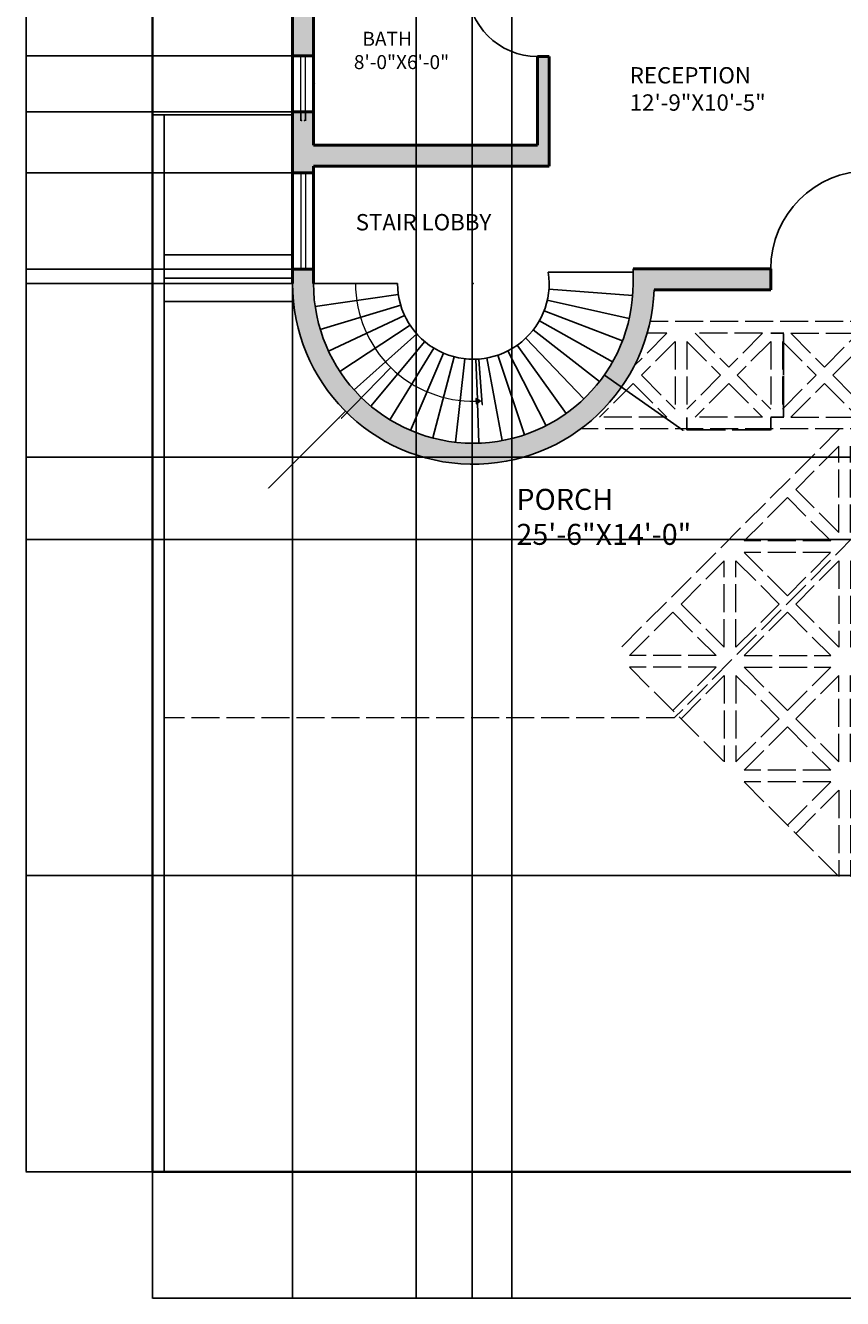
# Model space of a CAD drawing. Units: inches. Extents: x 2447 to 3157, y 2799 to 3988.
# Tile 1 of 9: x 2447 to 2797, y 2799 to 3345. Entities that reach past the tile are written whole.
import ezdxf

# ---------------------------------------------------------------- set-up
doc = ezdxf.new("R2010")
doc.units = ezdxf.units.IN
doc.linetypes.add('ACAD_ISO02W100', pattern=[15, 12, -3])
for name, color, linetype, lineweight in [('A-ANNO-DIMS', 2, 'Continuous', 18), ('A-ANNO-SYMB', 2, 'Continuous', 18), ('A-AREA-IDEN', 7, 'Continuous', 25), ('A-DOOR', 3, 'Continuous', 25), ('A-FLOR-OVHD', 8, 'ACAD_ISO02W100', 18), ('A-FLOR-STRS', 7, 'Continuous', 25), ('A-GLAZ', 4, 'Continuous', 18), ('A-WALL', 7, 'Continuous', 50), ('A-WALL-PATT', 252, 'Continuous', 13), ('C-PROP', 6, 'Continuous', 35), ('C-SITE', 8, 'Continuous', 25), ('L-PAVE-PATT', 9, 'ACAD_ISO02W100', 13)]:
    doc.layers.add(name, color=color, linetype=linetype, lineweight=lineweight)
doc.styles.get("Standard").update_dxf_attribs({"font": 'arial.ttf'})
doc.dimstyles.get("Standard").update_dxf_attribs({"dimtxt": 0.18, "dimasz": 0.18, "dimexe": 0.18, "dimexo": 0.0625, "dimgap": 0.09, "dimtad": 0, "dimtih": 1, "dimtoh": 1, "dimdec": 4, "dimzin": 0, "dimdsep": 46, "dimtxsty": 'Standard', "dimcen": 0.09, "dimadec": 0, "dimazin": 0, "dimtfac": 1, "dimtdec": 4, "dimtofl": 0, "dimtmove": 0, "dimatfit": 3, "dimfxl": 1, "dimtolj": 1, "dimtzin": 0, "dimarcsym": 0})

# ---------------------------------------------------------------- blocks, each defined once
blk = doc.blocks.new('DOOR-SWING-30IN')
for p, q in [((0, 1), (-29.98, 1)), ((0, 1), (0, 0)), ((0, 0), (-30, 0))]:
    blk.add_line(p, q)
blk.add_arc((0, 0), 30, 90, 180)
blk = doc.blocks.new('DOOR-SWING-42IN')
for p, q in [((0, 0), (0, 42)), ((1, 0), (1, 41.99)), ((1, 0), (0, 0))]:
    blk.add_line(p, q)
blk.add_arc((0, 0), 42, 0, 90)
blk = doc.blocks.new('GLAZING-24IN')
for p, q in [((0, 0), (0, 24)), ((2, 0), (2, 24))]:
    blk.add_line(p, q)
blk = doc.blocks.new('PAVER-PANEL-LINKED')
for p, q in [((0, 60.96), (0, 34.75)), ((26.22, 34.75), (0, 60.96)), ((60.97, 64.5), (3.54, 64.5)), ((29.75, 38.29), (3.54, 64.5)), ((29.75, 64.5), (29.75, 38.29)), ((34.75, 64.5), (34.75, 38.29)), ((34.75, 38.29), (60.97, 64.5)), ((38.29, 34.75), (64.51, 60.96)), ((64.51, 60.96), (64.51, 34.75)), ((26.22, 34.75), (0, 34.75)), ((64.51, 34.75), (38.29, 34.75)), ((0, 29.75), (0, 3.54)), ((26.22, 29.75), (0, 3.54)), ((26.22, 29.75), (0, 29.75)), ((64.51, 29.75), (38.29, 29.75)), ((38.29, 29.75), (64.51, 3.54)), ((64.51, 29.75), (64.51, 3.54)), ((29.75, 26.21), (3.54, 0)), ((29.75, 26.21), (29.75, 0)), ((34.75, 26.21), (34.75, 0)), ((34.75, 26.21), (60.97, 0)), ((29.75, 0), (3.54, 0)), ((60.97, 0), (34.75, 0))]:
    blk.add_line(p, q)
blk = doc.blocks.new('PORCH-PAVER-FOUR-TRIANGLE')
for p, q in [((32.46, 36), (3.54, 36)), ((3.54, 36), (18, 21.54)), ((32.46, 36), (18, 21.54)), ((0, 32.46), (0, 3.54)), ((0, 32.46), (14.46, 18)), ((36, 32.46), (21.54, 18)), ((36, 32.46), (36, 3.54)), ((14.46, 18), (0, 3.54)), ((21.54, 18), (36, 3.54)), ((18, 14.46), (3.54, 0)), ((18, 14.46), (32.46, 0)), ((32.46, 0), (3.54, 0))]:
    blk.add_line(p, q)
blk = doc.blocks.new('*D22')
at = {"layer": 'A-ANNO-DIMS', "color": 0, "lineweight": -2, "transparency": 16777216}
for p, q in [((2566.93, 3331.93), (2570.65, 3331.93)), ((2570.47, 3331.75), (2570.47, 3320.11)), ((2570.47, 3308.11), (2570.47, 3319.74)), ((2566.93, 3307.93), (2570.65, 3307.93))]:
    blk.add_line(p, q, dxfattribs=at)
at = {"layer": 'A-ANNO-DIMS', "color": 0, "transparency": 16777216}
for points in [[(2570.44, 3331.75), (2570.5, 3331.75), (2570.47, 3331.93)], [(2570.44, 3308.11), (2570.5, 3308.11), (2570.47, 3307.93)]]:
    blk.add_solid(points, dxfattribs=at)
at = {"layer": 'Defpoints', "color": 0, "transparency": 16777216}
for p in [(2566.87, 3331.93), (2570.47, 3331.93), (2566.87, 3307.93)]:
    blk.add_point(p, dxfattribs=at)
at = {"layer": 'A-ANNO-DIMS', "color": 0, "transparency": 16777216, "insert": (2570.47, 3319.93), "char_height": 0.18, "attachment_point": 5}
blk.add_mtext('\\A1;GLAZING 24 TYP.', dxfattribs=at)
blk = doc.blocks.new('*D23')
at = {"layer": 'A-ANNO-DIMS', "color": 0, "lineweight": -2, "transparency": 16777216}
for p, q in [((2564.87, 3307.87), (2564.87, 3304.15)), ((2566.87, 3307.87), (2566.87, 3304.15)), ((2565.05, 3304.33), (2565.41, 3304.33)), ((2566.69, 3304.33), (2566.33, 3304.33))]:
    blk.add_line(p, q, dxfattribs=at)
at = {"layer": 'A-ANNO-DIMS', "color": 0, "transparency": 16777216}
for points in [[(2565.05, 3304.36), (2565.05, 3304.3), (2564.87, 3304.33)], [(2566.69, 3304.36), (2566.69, 3304.3), (2566.87, 3304.33)]]:
    blk.add_solid(points, dxfattribs=at)
at = {"layer": 'Defpoints', "color": 0, "transparency": 16777216}
for p in [(2564.87, 3307.93), (2566.87, 3307.93), (2566.87, 3304.33)]:
    blk.add_point(p, dxfattribs=at)
at = {"layer": 'A-ANNO-DIMS', "color": 0, "transparency": 16777216, "insert": (2565.87, 3304.33), "char_height": 0.18, "attachment_point": 5}
blk.add_mtext('\\A1;2 TYP.', dxfattribs=at)
blk = doc.blocks.new('*D42')
at = {"layer": 'A-ANNO-DIMS', "color": 0, "lineweight": -2, "transparency": 16777216}
for p, q in [((2730.37, 3177.01), (2730.37, 3171.49)), ((2766.37, 3177.01), (2766.37, 3171.49)), ((2730.55, 3171.67), (2746.89, 3171.67)), ((2766.19, 3171.67), (2749.84, 3171.67))]:
    blk.add_line(p, q, dxfattribs=at)
at = {"layer": 'A-ANNO-DIMS', "color": 0, "transparency": 16777216}
for points in [[(2730.55, 3171.7), (2730.55, 3171.64), (2730.37, 3171.67)], [(2766.19, 3171.7), (2766.19, 3171.64), (2766.37, 3171.67)]]:
    blk.add_solid(points, dxfattribs=at)
at = {"layer": 'Defpoints', "color": 0, "transparency": 16777216}
for p in [(2730.37, 3177.07), (2766.37, 3177.07), (2766.37, 3171.67)]:
    blk.add_point(p, dxfattribs=at)
at = {"layer": 'A-ANNO-DIMS', "color": 0, "transparency": 16777216, "insert": (2748.37, 3171.67), "char_height": 0.18, "attachment_point": 5}
blk.add_mtext('\\A1;PORCH PAVER 36 TYP.', dxfattribs=at)
blk = doc.blocks.new('*D43')
at = {"layer": 'A-ANNO-DIMS', "color": 0, "lineweight": -2, "transparency": 16777216}
for p, q in [((2766.43, 3213.07), (2771.95, 3213.07)), ((2771.77, 3212.89), (2771.77, 3195.26)), ((2771.77, 3177.25), (2771.77, 3194.89)), ((2766.43, 3177.07), (2771.95, 3177.07))]:
    blk.add_line(p, q, dxfattribs=at)
at = {"layer": 'A-ANNO-DIMS', "color": 0, "transparency": 16777216}
for points in [[(2771.74, 3212.89), (2771.8, 3212.89), (2771.77, 3213.07)], [(2771.74, 3177.25), (2771.8, 3177.25), (2771.77, 3177.07)]]:
    blk.add_solid(points, dxfattribs=at)
at = {"layer": 'Defpoints', "color": 0, "transparency": 16777216}
for p in [(2766.37, 3213.07), (2771.77, 3213.07), (2766.37, 3177.07)]:
    blk.add_point(p, dxfattribs=at)
at = {"layer": 'A-ANNO-DIMS', "color": 0, "transparency": 16777216, "insert": (2771.77, 3195.07), "char_height": 0.18, "attachment_point": 5}
blk.add_mtext('\\A1;36 TYP.', dxfattribs=at)
blk = doc.blocks.new('*D44')
at = {"layer": 'A-ANNO-DIMS', "color": 0, "lineweight": -2, "transparency": 16777216}
for p, q in [((2501.37, 2853.64), (2501.37, 2799.37)), ((3102.37, 2853.64), (3102.37, 2799.37)), ((2501.55, 2799.55), (2801.6, 2799.55)), ((3102.19, 2799.55), (2802.14, 2799.55))]:
    blk.add_line(p, q, dxfattribs=at)
at = {"layer": 'A-ANNO-DIMS', "color": 0, "transparency": 16777216}
for points in [[(2501.55, 2799.58), (2501.55, 2799.52), (2501.37, 2799.55)], [(3102.19, 2799.58), (3102.19, 2799.52), (3102.37, 2799.55)]]:
    blk.add_solid(points, dxfattribs=at)
at = {"layer": 'Defpoints', "color": 0, "transparency": 16777216}
for p in [(2501.37, 2853.7), (3102.37, 2853.7), (3102.37, 2799.55)]:
    blk.add_point(p, dxfattribs=at)
at = {"layer": 'A-ANNO-DIMS', "color": 0, "transparency": 16777216, "insert": (2801.87, 2799.55), "char_height": 0.18, "attachment_point": 5}
blk.add_mtext('\\A1;601', dxfattribs=at)
blk = doc.blocks.new('*D45')
at = {"layer": 'A-ANNO-DIMS', "color": 0, "lineweight": -2, "transparency": 16777216}
for p, q in [((2501.3, 3933.7), (2447.04, 3933.7)), ((2447.22, 3933.52), (2447.22, 3393.88)), ((2447.22, 2853.88), (2447.22, 3393.52)), ((2501.3, 2853.7), (2447.04, 2853.7))]:
    blk.add_line(p, q, dxfattribs=at)
at = {"layer": 'A-ANNO-DIMS', "color": 0, "transparency": 16777216}
for points in [[(2447.19, 3933.52), (2447.25, 3933.52), (2447.22, 3933.7)], [(2447.19, 2853.88), (2447.25, 2853.88), (2447.22, 2853.7)]]:
    blk.add_solid(points, dxfattribs=at)
at = {"layer": 'Defpoints', "color": 0, "transparency": 16777216}
for p in [(2447.22, 3933.7), (2501.37, 3933.7), (2501.37, 2853.7)]:
    blk.add_point(p, dxfattribs=at)
at = {"layer": 'A-ANNO-DIMS', "color": 0, "transparency": 16777216, "insert": (2447.22, 3393.7), "char_height": 0.18, "attachment_point": 5}
blk.add_mtext('\\A1;1080', dxfattribs=at)
blk = doc.blocks.new('*D54')
at = {"layer": 'A-ANNO-DIMS', "color": 0, "lineweight": -2, "transparency": 16777216}
for p, q in [((2561.3, 3240.53), (2447.04, 3240.53)), ((2447.22, 3240.35), (2447.22, 3237.67)), ((2447.22, 3234.63), (2447.22, 3237.3)), ((2561.3, 3234.45), (2447.04, 3234.45))]:
    blk.add_line(p, q, dxfattribs=at)
at = {"layer": 'A-ANNO-DIMS', "color": 0, "transparency": 16777216}
for points in [[(2447.19, 3240.35), (2447.25, 3240.35), (2447.22, 3240.53)], [(2447.19, 3234.63), (2447.25, 3234.63), (2447.22, 3234.45)]]:
    blk.add_solid(points, dxfattribs=at)
at = {"layer": 'Defpoints', "color": 0, "transparency": 16777216}
for p in [(2447.22, 3240.53), (2561.37, 3240.53), (2561.37, 3234.45)]:
    blk.add_point(p, dxfattribs=at)
at = {"layer": 'A-ANNO-DIMS', "color": 0, "transparency": 16777216, "insert": (2447.22, 3237.49), "char_height": 0.18, "attachment_point": 5}
blk.add_mtext('\\A1;6.08', dxfattribs=at)
blk = doc.blocks.new('*D55')
at = {"layer": 'A-ANNO-DIMS', "color": 0, "lineweight": -2, "transparency": 16777216}
for p, q in [((2561.3, 3281.78), (2447.04, 3281.78)), ((2447.22, 3281.6), (2447.22, 3261.33)), ((2447.22, 3240.71), (2447.22, 3260.97)), ((2561.3, 3240.53), (2447.04, 3240.53))]:
    blk.add_line(p, q, dxfattribs=at)
at = {"layer": 'A-ANNO-DIMS', "color": 0, "transparency": 16777216}
for points in [[(2447.19, 3281.6), (2447.25, 3281.6), (2447.22, 3281.78)], [(2447.19, 3240.71), (2447.25, 3240.71), (2447.22, 3240.53)]]:
    blk.add_solid(points, dxfattribs=at)
at = {"layer": 'Defpoints', "color": 0, "transparency": 16777216}
for p in [(2447.22, 3281.78), (2561.37, 3281.78), (2561.37, 3240.53)]:
    blk.add_point(p, dxfattribs=at)
at = {"layer": 'A-ANNO-DIMS', "color": 0, "transparency": 16777216, "insert": (2447.22, 3261.15), "char_height": 0.18, "attachment_point": 5}
blk.add_mtext('\\A1;41.25', dxfattribs=at)
blk = doc.blocks.new('*D56')
at = {"layer": 'A-ANNO-DIMS', "color": 0, "lineweight": -2, "transparency": 16777216}
for p, q in [((2561.3, 3307.93), (2447.04, 3307.93)), ((2447.22, 3307.75), (2447.22, 3295.03)), ((2447.22, 3281.96), (2447.22, 3294.67)), ((2561.3, 3281.78), (2447.04, 3281.78))]:
    blk.add_line(p, q, dxfattribs=at)
at = {"layer": 'A-ANNO-DIMS', "color": 0, "transparency": 16777216}
for points in [[(2447.19, 3307.75), (2447.25, 3307.75), (2447.22, 3307.93)], [(2447.19, 3281.96), (2447.25, 3281.96), (2447.22, 3281.78)]]:
    blk.add_solid(points, dxfattribs=at)
at = {"layer": 'Defpoints', "color": 0, "transparency": 16777216}
for p in [(2447.22, 3307.93), (2561.37, 3307.93), (2561.37, 3281.78)]:
    blk.add_point(p, dxfattribs=at)
at = {"layer": 'A-ANNO-DIMS', "color": 0, "transparency": 16777216, "insert": (2447.22, 3294.85), "char_height": 0.18, "attachment_point": 5}
blk.add_mtext('\\A1;26.15', dxfattribs=at)
blk = doc.blocks.new('*D57')
at = {"layer": 'A-ANNO-DIMS', "color": 0, "lineweight": -2, "transparency": 16777216}
for p, q in [((2561.3, 3412.7), (2447.04, 3412.7)), ((2447.22, 3412.52), (2447.22, 3372.5)), ((2447.22, 3332.11), (2447.22, 3372.13)), ((2561.3, 3331.93), (2447.04, 3331.93))]:
    blk.add_line(p, q, dxfattribs=at)
at = {"layer": 'A-ANNO-DIMS', "color": 0, "transparency": 16777216}
for points in [[(2447.19, 3412.52), (2447.25, 3412.52), (2447.22, 3412.7)], [(2447.19, 3332.11), (2447.25, 3332.11), (2447.22, 3331.93)]]:
    blk.add_solid(points, dxfattribs=at)
at = {"layer": 'Defpoints', "color": 0, "transparency": 16777216}
for p in [(2447.22, 3412.7), (2561.37, 3412.7), (2561.37, 3331.93)]:
    blk.add_point(p, dxfattribs=at)
at = {"layer": 'A-ANNO-DIMS', "color": 0, "transparency": 16777216, "insert": (2447.22, 3372.31), "char_height": 0.18, "attachment_point": 5}
blk.add_mtext('\\A1;80.77', dxfattribs=at)
blk = doc.blocks.new('*D68')
at = {"layer": 'A-ANNO-DIMS', "color": 0, "lineweight": -2, "transparency": 16777216}
for p, q in [((2561.37, 3849.64), (2561.37, 2799.37)), ((2614.37, 3840.64), (2614.37, 2799.37)), ((2561.55, 2799.55), (2587.65, 2799.55)), ((2614.19, 2799.55), (2588.09, 2799.55))]:
    blk.add_line(p, q, dxfattribs=at)
at = {"layer": 'A-ANNO-DIMS', "color": 0, "transparency": 16777216}
for points in [[(2561.55, 2799.58), (2561.55, 2799.52), (2561.37, 2799.55)], [(2614.19, 2799.58), (2614.19, 2799.52), (2614.37, 2799.55)]]:
    blk.add_solid(points, dxfattribs=at)
at = {"layer": 'Defpoints', "color": 0, "transparency": 16777216}
for p in [(2561.37, 3849.7), (2614.37, 3840.7), (2614.37, 2799.55)]:
    blk.add_point(p, dxfattribs=at)
at = {"layer": 'A-ANNO-DIMS', "color": 0, "transparency": 16777216, "insert": (2587.87, 2799.55), "char_height": 0.18, "attachment_point": 5}
blk.add_mtext('\\A1;53', dxfattribs=at)
blk = doc.blocks.new('*D69')
at = {"layer": 'A-ANNO-DIMS', "color": 0, "lineweight": -2, "transparency": 16777216}
for p, q in [((2638.37, 3840.64), (2638.37, 2799.37)), ((2655.37, 3840.64), (2655.37, 2799.37)), ((2638.55, 2799.55), (2646.66, 2799.55)), ((2655.19, 2799.55), (2647.08, 2799.55))]:
    blk.add_line(p, q, dxfattribs=at)
at = {"layer": 'A-ANNO-DIMS', "color": 0, "transparency": 16777216}
for points in [[(2638.55, 2799.58), (2638.55, 2799.52), (2638.37, 2799.55)], [(2655.19, 2799.58), (2655.19, 2799.52), (2655.37, 2799.55)]]:
    blk.add_solid(points, dxfattribs=at)
at = {"layer": 'Defpoints', "color": 0, "transparency": 16777216}
for p in [(2638.37, 3840.7), (2655.37, 3840.7), (2655.37, 2799.55)]:
    blk.add_point(p, dxfattribs=at)
at = {"layer": 'A-ANNO-DIMS', "color": 0, "transparency": 16777216, "insert": (2646.87, 2799.55), "char_height": 0.18, "attachment_point": 5}
blk.add_mtext('\\A1;17', dxfattribs=at)
blk = doc.blocks.new('*D71')
at = {"layer": 'A-ANNO-DIMS', "color": 0, "lineweight": -2, "transparency": 16777216}
for p, q in [((3001.74, 2980.7), (2447.04, 2980.7)), ((2447.22, 2980.52), (2447.22, 2917.38)), ((2447.22, 2853.88), (2447.22, 2917.02)), ((3102.3, 2853.7), (2447.04, 2853.7))]:
    blk.add_line(p, q, dxfattribs=at)
at = {"layer": 'A-ANNO-DIMS', "color": 0, "transparency": 16777216}
for points in [[(2447.19, 2980.52), (2447.25, 2980.52), (2447.22, 2980.7)], [(2447.19, 2853.88), (2447.25, 2853.88), (2447.22, 2853.7)]]:
    blk.add_solid(points, dxfattribs=at)
at = {"layer": 'Defpoints', "color": 0, "transparency": 16777216}
for p in [(3001.81, 2980.7), (2447.22, 2853.7), (3102.37, 2853.7)]:
    blk.add_point(p, dxfattribs=at)
at = {"layer": 'A-ANNO-DIMS', "color": 0, "transparency": 16777216, "insert": (2447.22, 2917.2), "char_height": 0.18, "attachment_point": 5}
blk.add_mtext('\\A1;127', dxfattribs=at)
blk = doc.blocks.new('*D74')
at = {"layer": 'A-ANNO-DIMS', "color": 0, "lineweight": -2, "transparency": 16777216}
for p, q in [((2812.3, 3159.97), (2447.04, 3159.97)), ((2447.22, 3159.79), (2447.22, 3142.52)), ((2447.22, 3124.88), (2447.22, 3142.15)), ((2847.58, 3124.7), (2447.04, 3124.7))]:
    blk.add_line(p, q, dxfattribs=at)
at = {"layer": 'A-ANNO-DIMS', "color": 0, "transparency": 16777216}
for points in [[(2447.19, 3159.79), (2447.25, 3159.79), (2447.22, 3159.97)], [(2447.19, 3124.88), (2447.25, 3124.88), (2447.22, 3124.7)]]:
    blk.add_solid(points, dxfattribs=at)
at = {"layer": 'Defpoints', "color": 0, "transparency": 16777216}
for p in [(2812.37, 3159.97), (2447.22, 3124.7), (2847.64, 3124.7)]:
    blk.add_point(p, dxfattribs=at)
at = {"layer": 'A-ANNO-DIMS', "color": 0, "transparency": 16777216, "insert": (2447.22, 3142.34), "char_height": 0.18, "attachment_point": 5}
blk.add_mtext('\\A1;35.27', dxfattribs=at)
blk = doc.blocks.new('*D77')
at = {"layer": 'A-ANNO-DIMS', "color": 0, "lineweight": -2, "transparency": 16777216}
for p, q in [((2638.78, 3234.45), (2638.96, 3234.45)), ((2638.87, 3234.36), (2638.87, 3234.54)), ((2551.19, 3146.76), (2583.94, 3179.52)), ((2551.01, 3146.76), (2551.19, 3146.76))]:
    blk.add_line(p, q, dxfattribs=at)
at = {"layer": 'A-ANNO-DIMS', "color": 0, "transparency": 16777216}
blk.add_solid([(2583.92, 3179.54), (2583.96, 3179.5), (2584.07, 3179.65)], dxfattribs=at)
at = {"layer": 'Defpoints', "color": 0, "transparency": 16777216}
for p in [(2638.87, 3234.45), (2584.07, 3179.65)]:
    blk.add_point(p, dxfattribs=at)
at = {"layer": 'A-ANNO-DIMS', "color": 0, "transparency": 16777216, "insert": (2550.6, 3146.76), "char_height": 0.18, "attachment_point": 5}
blk.add_mtext('\\A1;R77.5', dxfattribs=at)
blk = doc.blocks.new('*D78')
at = {"layer": 'A-ANNO-DIMS', "color": 0, "lineweight": -2, "transparency": 16777216}
for p, q in [((2638.78, 3234.45), (2638.96, 3234.45)), ((2638.87, 3234.36), (2638.87, 3234.54)), ((2728.64, 3171.58), (2695.12, 3195.05)), ((2728.82, 3171.58), (2728.64, 3171.58))]:
    blk.add_line(p, q, dxfattribs=at)
at = {"layer": 'A-ANNO-DIMS', "color": 0, "transparency": 16777216}
blk.add_solid([(2695.14, 3195.07), (2695.11, 3195.02), (2694.98, 3195.15)], dxfattribs=at)
at = {"layer": 'Defpoints', "color": 0, "transparency": 16777216}
for p in [(2638.87, 3234.45), (2694.98, 3195.15)]:
    blk.add_point(p, dxfattribs=at)
at = {"layer": 'A-ANNO-DIMS', "color": 0, "transparency": 16777216, "insert": (2729.23, 3171.58), "char_height": 0.18, "attachment_point": 5}
blk.add_mtext('\\A1;R68.5', dxfattribs=at)
blk = doc.blocks.new('*D79')
at = {"layer": 'A-ANNO-DIMS', "color": 0, "lineweight": -2, "transparency": 16777216}
for p, q in [((2638.78, 3234.45), (2638.96, 3234.45)), ((2638.87, 3234.36), (2638.87, 3234.54)), ((2582.37, 3176.68), (2603.43, 3198.22)), ((2582.19, 3176.68), (2582.37, 3176.68))]:
    blk.add_line(p, q, dxfattribs=at)
at = {"layer": 'A-ANNO-DIMS', "color": 0, "transparency": 16777216}
blk.add_solid([(2603.41, 3198.24), (2603.45, 3198.2), (2603.56, 3198.35)], dxfattribs=at)
at = {"layer": 'Defpoints', "color": 0, "transparency": 16777216}
for p in [(2638.87, 3234.45), (2603.56, 3198.35)]:
    blk.add_point(p, dxfattribs=at)
at = {"layer": 'A-ANNO-DIMS', "color": 0, "transparency": 16777216, "insert": (2581.78, 3176.68), "char_height": 0.18, "attachment_point": 5}
blk.add_mtext('\\A1;R50.5', dxfattribs=at)
blk = doc.blocks.new('*D80')
at = {"layer": 'A-ANNO-DIMS', "color": 0, "lineweight": -2, "transparency": 16777216}
for p, q in [((2638.78, 3234.45), (2638.96, 3234.45)), ((2638.87, 3234.36), (2638.87, 3234.54)), ((2642.72, 3182.59), (2641.29, 3201.86)), ((2642.9, 3182.59), (2642.72, 3182.59))]:
    blk.add_line(p, q, dxfattribs=at)
at = {"layer": 'A-ANNO-DIMS', "color": 0, "transparency": 16777216}
blk.add_solid([(2641.32, 3201.86), (2641.26, 3201.85), (2641.27, 3202.04)], dxfattribs=at)
at = {"layer": 'Defpoints', "color": 0, "transparency": 16777216}
for p in [(2638.87, 3234.45), (2641.27, 3202.04)]:
    blk.add_point(p, dxfattribs=at)
at = {"layer": 'A-ANNO-DIMS', "color": 0, "transparency": 16777216, "insert": (2643.31, 3182.59), "char_height": 0.18, "attachment_point": 5}
blk.add_mtext('\\A1;R32.5', dxfattribs=at)

msp = doc.modelspace()

# ---------------------------------------------------------------- hatches: boundary and pattern name
at = {"layer": 'A-ANNO-SYMB'}
h = msp.add_hatch(color=256, dxfattribs=at)
h.dxf.hatch_style = 1
h.paths.add_polyline_path([(2641.9403, 3184.0566), (2639.9163, 3185.0672), (2640.0531, 3182.8091)])
at = {"layer": 'A-WALL-PATT'}
h = msp.add_hatch(color=256, dxfattribs=at)
h.dxf.hatch_style = 1
h.paths.add_polyline_path([(2570.3672, 3550.7002), (2726.3672, 3550.7002), (2726.3672, 3370.7002), (2722.3672, 3370.7002), (2722.3672, 3365.7002), (2739.3672, 3365.7002), (2739.3672, 3374.7002), (2735.3672, 3374.7002), (2735.3672, 3563.7002), (2726.3672, 3563.7002), (2726.3672, 3559.7002), (2570.3672, 3559.7002), (2570.3672, 3599.2479), (2561.3672, 3599.2479), (2561.3672, 3508.7002), (2570.3672, 3508.7002)])
h.paths.add_polyline_path([(2570.3672, 3412.7002), (2561.3672, 3412.7002), (2561.3672, 3331.9279), (2570.3672, 3331.9279), (2570.3672, 3365.7002), (2666.3672, 3365.7002), (2666.3672, 3361.7002), (2671.3672, 3361.7002), (2671.3672, 3365.7002), (2686.3672, 3365.7002), (2686.3672, 3370.7002), (2570.3672, 3370.7002)])
h.paths.add_polyline_path([(2965.3672, 3430.7002), (2961.3672, 3430.7002), (2961.3672, 3434.7002), (2952.3672, 3434.7002), (2952.3672, 3430.7002), (2847.6393, 3430.7002), (2812.3672, 3395.4282), (2812.3672, 3374.7002), (2781.3672, 3374.7002), (2781.3672, 3365.7002), (2812.3672, 3365.7002), (2812.3672, 3347.7002), (2821.3672, 3347.7002), (2821.3672, 3391.7002), (2851.3672, 3421.7002), (2965.3672, 3421.7002)])
h.paths.add_polyline_path([(3046.3672, 3430.7002), (3033.3672, 3430.7002), (3033.3672, 3421.7002), (3037.3672, 3421.7002), (3037.3672, 3133.7002), (2971.1661, 3133.7002), (2971.1661, 3124.7002), (3046.3672, 3124.7002)])
h.paths.add_polyline_path([(3046.3672, 3825.7002), (3005.5801, 3825.7002), (3005.5801, 3816.7002), (3037.3672, 3816.7002), (3037.3672, 3655.7002), (2940.3672, 3655.7002), (2940.3672, 3646.7002), (3037.3672, 3646.7002), (3037.3672, 3514.7002), (3033.3672, 3514.7002), (3033.3672, 3505.7002), (3046.3672, 3505.7002)])
h.paths.add_polyline_path([(2821.3672, 3258.7002), (2812.3672, 3258.7002), (2812.3672, 3240.7002), (2808.3672, 3240.7002), (2808.3672, 3231.7002), (2812.3672, 3231.7002), (2812.3672, 3223.0688), (2821.3672, 3223.0688)])
h.paths.add_polyline_path([(2766.3672, 3240.7002), (2707.3672, 3240.7002), (2707.3672, 3234.4466, -1), (2570.3672, 3234.4466), (2570.3672, 3240.5271), (2561.3672, 3240.5271), (2561.3672, 3234.4466, 0.98243292), (2716.3185, 3231.7002), (2766.3672, 3231.7002)])
h.paths.add_polyline_path([(2570.3672, 3307.9279), (2561.3672, 3307.9279), (2561.3672, 3281.7773), (2570.3672, 3281.7773), (2570.3672, 3284.7002), (2671.3672, 3284.7002), (2671.3672, 3331.7002), (2666.3672, 3331.7002), (2666.3672, 3293.7002), (2570.3672, 3293.7002)])
h.paths.add_polyline_path([(2570.3672, 3739.7002), (2574.3672, 3739.7002), (2574.3672, 3744.7002), (2570.3672, 3744.7002), (2570.3672, 3840.7002), (2614.3672, 3840.7002), (2614.3672, 3849.7002), (2561.3672, 3849.7002), (2561.3672, 3671.2479), (2570.3672, 3671.2479)])
h.paths.add_polyline_path([(2735.3672, 3840.7002), (2789.3672, 3840.7002), (2789.3672, 3816.7002), (2798.3672, 3816.7002), (2798.3672, 3849.7002), (2679.3672, 3849.7002), (2679.3672, 3840.7002), (2726.3672, 3840.7002), (2726.3672, 3778.7002), (2735.3672, 3778.7002)])
h.paths.add_polyline_path([(2651.3672, 3840.7002), (2655.3672, 3840.7002), (2655.3672, 3849.7002), (2638.3672, 3849.7002), (2638.3672, 3840.7002), (2642.3672, 3840.7002), (2642.3672, 3744.7002), (2610.3672, 3744.7002), (2610.3672, 3739.7002), (2726.3672, 3739.7002), (2726.3672, 3599.7002), (2735.3672, 3599.7002), (2735.3672, 3622.7002), (2739.3672, 3622.7002), (2739.3672, 3631.7002), (2735.3672, 3631.7002), (2735.3672, 3748.7002), (2726.3672, 3748.7002), (2726.3672, 3744.7002), (2651.3672, 3744.7002)])
h.paths.add_polyline_path([(2900.3672, 3816.7002), (2904.3672, 3816.7002), (2904.3672, 3825.7002), (2882.3672, 3825.7002), (2882.3672, 3816.7002), (2891.3672, 3816.7002), (2891.3672, 3650.4282), (2872.6393, 3631.7002), (2775.3672, 3631.7002), (2775.3672, 3622.7002), (2876.3672, 3622.7002), (2900.3672, 3646.7002), (2904.3672, 3646.7002), (2904.3672, 3655.7002), (2900.3672, 3655.7002)])
h.paths.add_polyline_path([(2957.5801, 3825.7002), (2940.3672, 3825.7002), (2940.3672, 3816.7002), (2957.5801, 3816.7002)], flags=17)

# ---------------------------------------------------------------- linework, layer by layer
at = {"layer": 'A-ANNO-SYMB'}
msp.add_lwpolyline([(2588.3672, 3234.4466, 0.42070274), (2639.9834, 3183.959, 0.42070274)], format="xyb", dxfattribs=at)
msp.add_lwpolyline([(2641.9403, 3184.0566), (2639.9163, 3185.0672), (2640.0531, 3182.8091)], close=True, dxfattribs=at)
at = {"layer": 'A-FLOR-OVHD'}
for p, q in [((2823.6143, 3147.799), (2725.011, 3048.248)), ((2725.011, 3048.248), (2506.3672, 3048.248))]:
    msp.add_line(p, q, dxfattribs=at)
at = {"layer": 'A-FLOR-STRS'}
for p, q in [((2506.3672, 3246.7256), (2561.3672, 3246.7256)), ((2506.3672, 3236.7256), (2561.3672, 3236.7256)), ((2671.0107, 3239.2475), (2707.3672, 3239.2475)), ((2606.3672, 3234.4466), (2570.3672, 3234.4466)), ((2671.2737, 3231.9823), (2707.17, 3229.2525)), ((2506.3672, 3226.7256), (2561.7528, 3226.7256)), ((2606.7129, 3229.7189), (2571.0959, 3224.4821)), ((2607.7427, 3225.0918), (2573.2663, 3214.7296)), ((2670.5705, 3227.2944), (2705.6879, 3219.3719)), ((2609.4346, 3220.6637), (2576.8322, 3205.3965)), ((2669.1928, 3222.7587), (2702.7843, 3209.812)), ((2611.7526, 3216.5288), (2581.7179, 3196.6814)), ((2664.5451, 3214.5244), (2692.9884, 3192.4567)), ((2667.17, 3218.4716), (2698.5209, 3200.7762)), ((2614.6475, 3212.7751), (2587.8194, 3188.7698)), ((2618.0576, 3209.4825), (2595.0069, 3181.8299)), ((2661.374, 3211.001), (2686.3045, 3185.0305)), ((2621.9104, 3206.7209), (2603.1275, 3176.0093)), ((2626.124, 3204.5491), (2612.0084, 3171.4319)), ((2630.6086, 3203.0134), (2621.4607, 3168.1951)), ((2649.3068, 3203.6689), (2660.8706, 3169.5767)), ((2653.6729, 3205.5149), (2670.073, 3173.4675)), ((2657.724, 3207.9764), (2678.6115, 3178.6556)), ((2635.269, 3202.1464), (2631.2833, 3166.3677)), ((2640.0059, 3201.9666), (2640.6105, 3184.7206)), ((2644.7186, 3202.4777), (2651.2001, 3167.066)), ((2640.6634, 3183.2125), (2641.2672, 3165.9887))]:
    msp.add_line(p, q, dxfattribs=at)
msp.add_lwpolyline([(2570.3672, 3234.4466, 1), (2707.3672, 3234.4466), (2707.3672, 3240.7002)], format="xyb", dxfattribs=at)
for radius, end in [(32.5, 8.494826), (77.5, 357.969176)]:
    msp.add_arc((2638.8672, 3234.4466), radius, 180, end, dxfattribs=at)
at = {"layer": 'A-GLAZ'}
for p, q in [((2564.8672, 3281.7773), (2564.8672, 3240.5271)), ((2566.8672, 3281.7773), (2566.8672, 3240.5271))]:
    msp.add_line(p, q, dxfattribs=at)
at = {"layer": 'A-WALL'}
for p, q in [((2561.3672, 3849.7002), (2561.3672, 3234.4466)), ((2570.3672, 3365.7002), (2570.3672, 3293.7002)), ((2561.3672, 3331.9279), (2570.3672, 3331.9279)), ((2666.3672, 3331.7002), (2671.3672, 3331.7002)), ((2666.3672, 3331.7002), (2666.3672, 3293.7002)), ((2671.3672, 3331.7002), (2671.3672, 3284.7002)), ((2561.3672, 3307.9279), (2570.3672, 3307.9279)), ((2570.3672, 3293.7002), (2666.3672, 3293.7002)), ((2570.3672, 3284.7002), (2671.3672, 3284.7002)), ((2570.3672, 3284.7002), (2570.3672, 3234.4466)), ((2570.3672, 3281.7773), (2561.3672, 3281.7773)), ((2570.3672, 3240.5271), (2561.3672, 3240.5271)), ((2707.3672, 3240.7002), (2766.3672, 3240.7002)), ((2766.3672, 3240.7002), (2766.3672, 3231.7002)), ((2716.3185, 3231.7002), (2766.3672, 3231.7002))]:
    msp.add_line(p, q, dxfattribs=at)
at = {"layer": 'C-PROP'}
for p, q in [((2501.3672, 3933.7002), (2501.3672, 2853.7002)), ((2501.3672, 2853.7002), (3102.3672, 2853.7002))]:
    msp.add_line(p, q, dxfattribs=at)
at = {"layer": 'C-SITE'}
for p, q in [((2501.3672, 3306.7256), (2561.3672, 3306.7256)), ((2506.3672, 3306.7256), (2506.3672, 2853.7002))]:
    msp.add_line(p, q, dxfattribs=at)
at = {"layer": 'L-PAVE-PATT'}
for p, q in [((2812.3672, 3218.0737), (2714.618, 3218.0737)), ((2721.8317, 3213.0737), (2707.8155, 3199.0575)), ((2725.3672, 3209.5382), (2710.9028, 3195.0737)), ((2721.8317, 3213.0737), (2713.3619, 3213.0737)), ((2725.3672, 3209.5382), (2725.3672, 3180.6093)), ((2710.9028, 3195.0737), (2725.3672, 3180.6093)), ((2707.3672, 3191.5382), (2692.9028, 3177.0737)), ((2707.3672, 3191.5382), (2721.8317, 3177.0737)), ((2721.8317, 3177.0737), (2692.9028, 3177.0737)), ((2812.3672, 3172.0737), (2684.8659, 3172.0737)), ((2795.8658, 3172.0737), (2702.2778, 3078.4857))]:
    msp.add_line(p, q, dxfattribs=at)

# ---------------------------------------------------------------- block references
at = {"layer": 'A-DOOR', "extrusion": (0, 0, -1), "zscale": -1, "rotation": 180}
msp.add_blockref('DOOR-SWING-30IN', (-2666.3672, 3361.7002), dxfattribs=at)
at = {"layer": 'A-DOOR', "extrusion": (0, 0, -1), "zscale": -1}
msp.add_blockref('DOOR-SWING-42IN', (-2808.3672, 3240.7002), dxfattribs=at)
at = {"layer": 'A-GLAZ'}
msp.add_blockref('GLAZING-24IN', (2564.8672, 3307.9279), dxfattribs=at)
at = {"layer": 'L-PAVE-PATT'}
msp.add_blockref('PORCH-PAVER-FOUR-TRIANGLE', (2730.367, 3177.074), dxfattribs=at)
for name, p, rotation in [('PORCH-PAVER-FOUR-TRIANGLE', (2807.367, 3177.0735), 89.99999999999523), ('PAVER-PANEL-LINKED', (2752.4576, 3121.5938), 315.0000000000008), ('PAVER-PANEL-LINKED', (2794.5361, 3072.4449), 134.9999999999991), ('PAVER-PANEL-LINKED', (2843.686, 3023.295), 134.9999999999991)]:
    msp.add_blockref(name, p, dxfattribs=dict(at, rotation=rotation))

# ---------------------------------------------------------------- texts
at = {"layer": 'A-AREA-IDEN', "attachment_point": 1}
for s, width, insert, char_height in [('  BATH\\P8\'-0"X6\'-0"', 49.614473, (2587.6574, 3342.2892), 6), ('RECEPTION\\P12\'-9"X10\'-5"', 100.524075, (2705.9176, 3327.1376), 7), ('\\pxt18;STAIR LOBBY', 93.457402, (2588.4598, 3264.1693), 7), ('PORCH\\P25\'-6"X14\'-0"', 45.968833, (2657.3495, 3146.3938), 9)]:
    msp.add_mtext_dynamic_manual_height_columns(s, width=width, gutter_width=12.5, heights=[0], dxfattribs=dict(at, insert=insert, char_height=char_height))

# ---------------------------------------------------------------- dimensions: what is measured, and where the dimension line sits
at = {"layer": 'A-ANNO-DIMS'}
for base, p1, p2, override, picture, middle in [((2447.2172, 3933.7002), (2501.3672, 2853.7002), (2501.3672, 3933.7002), {"dimdec": 0, "dimlfac": 1, "dimrnd": 0, "dimzin": 0, "dimdsep": 46, "dimlunit": 2}, '*D45', (2447.2172, 3393.7002)), ((2447.2172, 3412.7002), (2561.3672, 3331.9279), (2561.3672, 3412.7002), {"dimdec": 2, "dimlfac": 1, "dimrnd": 0, "dimzin": 0, "dimdsep": 46, "dimlunit": 2}, '*D57', (2447.2172, 3372.3141)), ((2447.2172, 3307.9279), (2561.3672, 3281.7773), (2561.3672, 3307.9279), {"dimdec": 2, "dimlfac": 1, "dimrnd": 0, "dimzin": 0, "dimdsep": 46, "dimlunit": 2}, '*D56', (2447.2172, 3294.8526)), ((2447.2172, 3281.7773), (2561.3672, 3240.5271), (2561.3672, 3281.7773), {"dimdec": 2, "dimlfac": 1, "dimrnd": 0, "dimzin": 0, "dimdsep": 46, "dimlunit": 2}, '*D55', (2447.2172, 3261.1522)), ((2447.2172, 3240.5271), (2561.3672, 3234.4466), (2561.3672, 3240.5271), {"dimdec": 2, "dimlfac": 1, "dimrnd": 0, "dimzin": 0, "dimdsep": 46, "dimlunit": 2}, '*D54', (2447.2172, 3237.4869)), ((2447.2172, 3124.7002), (2812.3672, 3159.9723), (2847.6393, 3124.7002), {"dimdec": 2, "dimlfac": 1, "dimrnd": 0, "dimzin": 0, "dimdsep": 46, "dimlunit": 2}, '*D74', (2447.2172, 3142.3363)), ((2447.2172, 2853.7002), (3001.807, 2980.7002), (3102.3672, 2853.7002), {"dimdec": 0, "dimlfac": 1, "dimrnd": 0, "dimzin": 0, "dimdsep": 46, "dimlunit": 2}, '*D71', (2447.2172, 2917.2002))]:
    dim = msp.add_linear_dim(base=base, p1=p1, p2=p2, angle=90, dimstyle='Standard', override=override, dxfattribs=at)
    dim.commit()
    dim.dimension.update_dxf_attribs({"geometry": picture, "text_midpoint": middle})
for base, p1, p2, picture, middle in [((2614.3672, 2799.5502), (2561.3672, 3849.7002), (2614.3672, 3840.7002), '*D68', (2587.8672, 2799.5502)), ((2655.3672, 2799.5502), (2638.3672, 3840.7002), (2655.3672, 3840.7002), '*D69', (2646.8672, 2799.5502)), ((3102.3672, 2799.5502), (2501.3672, 2853.7002), (3102.3672, 2853.7002), '*D44', (2801.8672, 2799.5502))]:
    dim = msp.add_linear_dim(base=base, p1=p1, p2=p2, dimstyle='Standard', override={"dimdec": 0, "dimlfac": 1, "dimrnd": 0, "dimzin": 0, "dimdsep": 46, "dimlunit": 2}, dxfattribs=at)
    dim.commit()
    dim.dimension.update_dxf_attribs({"geometry": picture, "text_midpoint": middle})
for base, p1, p2, text, picture, middle in [((2570.4672, 3331.9279), (2566.8672, 3307.9279), (2566.8672, 3331.9279), 'GLAZING <> TYP.', '*D22', (2570.4672, 3319.9279)), ((2771.7672, 3213.0737), (2766.3672, 3177.0737), (2766.3672, 3213.0737), '<> TYP.', '*D43', (2771.7672, 3195.0737))]:
    dim = msp.add_linear_dim(base=base, p1=p1, p2=p2, angle=90, text=text, dimstyle='Standard', override={"dimdec": 0, "dimlfac": 1, "dimrnd": 0, "dimzin": 0, "dimdsep": 46, "dimlunit": 2}, dxfattribs=at)
    dim.commit()
    dim.dimension.update_dxf_attribs({"geometry": picture, "text_midpoint": middle})
for base, p1, p2, text, picture, middle in [((2566.8672, 3304.3279), (2564.8672, 3307.9279), (2566.8672, 3307.9279), '<> TYP.', '*D23', (2565.8672, 3304.3279)), ((2766.3672, 3171.6737), (2730.3672, 3177.0737), (2766.3672, 3177.0737), 'PORCH PAVER <> TYP.', '*D42', (2748.3672, 3171.6737))]:
    dim = msp.add_linear_dim(base=base, p1=p1, p2=p2, text=text, dimstyle='Standard', override={"dimdec": 0, "dimlfac": 1, "dimrnd": 0, "dimzin": 0, "dimdsep": 46, "dimlunit": 2}, dxfattribs=at)
    dim.commit()
    dim.dimension.update_dxf_attribs({"geometry": picture, "text_midpoint": middle})
for mpoint, picture, middle in [((2584.0671, 3179.6451), '*D77', (2550.5965, 3146.7643)), ((2603.5552, 3198.3452), '*D79', (2581.7774, 3176.6844)), ((2694.9764, 3195.1528), '*D78', (2729.2326, 3171.5765)), ((2641.274, 3202.0359), '*D80', (2643.3087, 3182.5894))]:
    dim = msp.add_radius_dim(center=(2638.8672, 3234.4466), mpoint=mpoint, dimstyle='Standard', override={"dimdec": 1, "dimlfac": 1, "dimrnd": 0, "dimzin": 0, "dimdsep": 46, "dimlunit": 2}, dxfattribs=at)
    dim.commit()
    dim.dimension.update_dxf_attribs({"geometry": picture, "text_midpoint": middle, "dimtype": 164})

doc.saveas('drawing.dxf')
